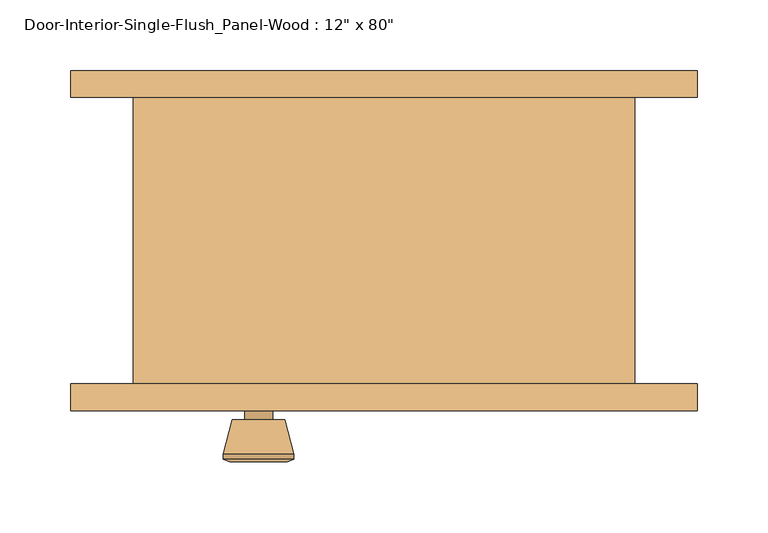
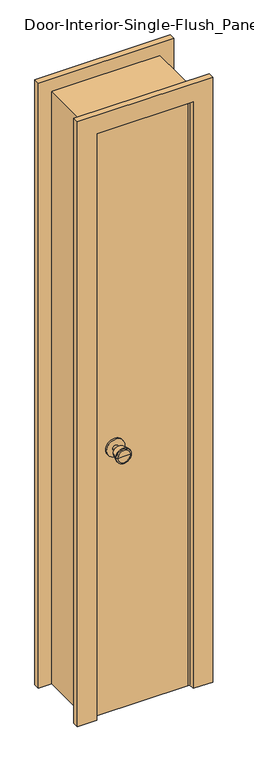
"""IFC4 building model written with IfcOpenShell, lengths in millimetres: door geometry."""

from ifc_helpers import new_model, si_unit, point, frame, frame_2d, origin, origin_with_axes, place, context, project, spatial, polyline, circle_curve, trimmed, segment, composite_curve, outline, extrude, faceted_brep, source, transform, mapped, element, save
from ifc_brep_helpers import plane_surface, cylinder_surface, revolved_surface, advanced_brep


def door_21b72c96(model_context):
    return source(origin(), model_context, "Body", "SolidModel", [
        advanced_brep(
        [(-88.9, -57.5, 914.4), (-98.9, -57.5, 914.4), (-78.9, -57.5, 914.4), (-68.4241324, -8.5, 914.4), (-109.3758676, -8.5, 914.4), (-88.9, -8.5, 914.4), (-63.9, -10.3278681, 914.4), (-113.9, -10.3278681, 914.4), (-63.9, -13.7915463, 914.4), (-113.9, -13.7915463, 914.4), (-70.263764, -38.5, 914.4), (-107.536236, -38.5, 914.4), (-78.9, -38.5, 914.4), (-98.9, -38.5, 914.4)],
        [
            (0, 1),
            (1, 2, circle_curve(frame((-88.9, -57.5, 914.4), z_axis=(0.0, -1.0, 0.0), x_axis=(-1.0, 0.0, 0.0)), 10.0)),
            (2, 0),
            (2, 1, circle_curve(frame((-88.9, -57.5, 914.4), z_axis=(0.0, -1.0, 0.0), x_axis=(-1.0, 0.0, 0.0)), 10.0)),
            (3, 4, circle_curve(frame((-88.9, -8.5, 914.4), z_axis=(0.0, 1.0, 0.0), x_axis=(-1.0, 0.0, 0.0)), 20.4758676)),
            (4, 5),
            (5, 3),
            (4, 3, circle_curve(frame((-88.9, -8.5, 914.4), z_axis=(0.0, 1.0, 0.0), x_axis=(-1.0, 0.0, 0.0)), 20.4758676)),
            (6, 7, circle_curve(frame((-88.9, -10.3278681, 914.4), z_axis=(0.0, 1.0, 0.0), x_axis=(-1.0, 0.0, 0.0)), 25.0)),
            (7, 4),
            (3, 6),
            (7, 6, circle_curve(frame((-88.9, -10.3278681, 914.4), z_axis=(0.0, 1.0, 0.0), x_axis=(-1.0, 0.0, 0.0)), 25.0)),
            (8, 9, circle_curve(frame((-88.9, -13.7915463, 914.4), z_axis=(0.0, 1.0, 0.0), x_axis=(-1.0, 0.0, 0.0)), 25.0)),
            (9, 7),
            (6, 8),
            (9, 8, circle_curve(frame((-88.9, -13.7915463, 914.4), z_axis=(0.0, 1.0, 0.0), x_axis=(-1.0, 0.0, 0.0)), 25.0)),
            (10, 11, circle_curve(frame((-88.9, -38.5, 914.4), z_axis=(0.0, 1.0, 0.0), x_axis=(-1.0, 0.0, 0.0)), 18.636236)),
            (11, 9),
            (8, 10),
            (11, 10, circle_curve(frame((-88.9, -38.5, 914.4), z_axis=(0.0, 1.0, 0.0), x_axis=(-1.0, 0.0, 0.0)), 18.636236)),
            (12, 13, circle_curve(frame((-88.9, -38.5, 914.4), z_axis=(0.0, 1.0, 0.0), x_axis=(-1.0, 0.0, 0.0)), 10.0)),
            (13, 11),
            (10, 12),
            (13, 12, circle_curve(frame((-88.9, -38.5, 914.4), z_axis=(0.0, 1.0, 0.0), x_axis=(-1.0, 0.0, 0.0)), 10.0)),
            (1, 13),
            (12, 2),
        ],
        [
            plane_surface(frame((-88.9, -57.5, 914.4), z_axis=(0.0, -1.0, 0.0), x_axis=(-1.0, 0.0, 0.0))),
            plane_surface(frame((-88.9, -8.5, 914.4), z_axis=(0.0, 1.0, 0.0), x_axis=(-1.0, 0.0, 0.0))),
            revolved_surface(polyline([(-109.3758676, -8.5, 914.4), (-113.9, -10.3278681, 914.4)]), (-88.9, -57.5, 914.4), (0.0, -1.0, 0.0)),
            cylinder_surface(frame((-88.9, -57.5, 914.4), z_axis=(0.0, -1.0, 0.0), x_axis=(-1.0, 0.0, 0.0)), 25.0),
            revolved_surface(polyline([(-113.9, -13.7915463, 914.4), (-107.536236, -38.5, 914.4)]), (-88.9, -57.5, 914.4), (0.0, -1.0, 0.0)),
            plane_surface(frame((-88.9, -38.5, 914.4), z_axis=(0.0, -1.0, 0.0), x_axis=(-1.0, 0.0, 0.0))),
            cylinder_surface(frame((-88.9, -57.5, 914.4), z_axis=(0.0, -1.0, 0.0), x_axis=(-1.0, 0.0, 0.0)), 10.0),
        ],
        [
            (0, [[1, 2, 3]]),
            (0, [[-3, 4, -1]]),
            (1, [[5, 6, 7]]),
            (1, [[8, -7, -6]]),
            (2, [[9, 10, -5, 11]]),
            (2, [[12, -11, -8, -10]]),
            (3, [[13, 14, -9, 15]]),
            (3, [[16, -15, -12, -14]]),
            (4, [[17, 18, -13, 19]]),
            (4, [[20, -19, -16, -18]]),
            (5, [[21, 22, -17, 23]]),
            (5, [[24, -23, -20, -22]]),
            (6, [[-2, 25, -21, 26]]),
            (6, [[-4, -26, -24, -25]]),
        ],
    ),
        extrude(outline(composite_curve([segment(trimmed(circle_curve(frame_2d((914.4, -88.9)), 30.0), [point((914.4, -118.9))], [point((914.4, -58.9))], False, "CARTESIAN"), True, "CONTINUOUS"), segment(trimmed(circle_curve(frame_2d((914.4, -88.9)), 30.0), [point((914.4, -58.9))], [point((914.4, -118.9))], False, "CARTESIAN"), True, "CONTINUOUS")], self_intersect=False)), frame((0.0, -63.5, 0.0), z_axis=(0.0, 1.0, 0.0), x_axis=(0.0, 0.0, 1.0)), (0.0, 0.0, 1.0), 6.0),
        advanced_brep(
        [(-88.9, -104.425, 914.4), (-78.9, -104.425, 914.4), (-98.9, -104.425, 914.4), (-68.4241324, -153.425, 914.4), (-88.9, -153.425, 914.4), (-109.3758676, -153.425, 914.4), (-63.9, -151.5971319, 914.4), (-113.9, -151.5971319, 914.4), (-63.9, -148.1334537, 914.4), (-113.9, -148.1334537, 914.4), (-70.263764, -123.425, 914.4), (-107.536236, -123.425, 914.4), (-78.9, -123.425, 914.4), (-98.9, -123.425, 914.4)],
        [
            (0, 1),
            (1, 2, circle_curve(frame((-88.9, -104.425, 914.4), z_axis=(0.0, 1.0, 0.0), x_axis=(-1.0, 0.0, 0.0)), 10.0)),
            (2, 0),
            (2, 1, circle_curve(frame((-88.9, -104.425, 914.4), z_axis=(0.0, 1.0, 0.0), x_axis=(-1.0, 0.0, 0.0)), 10.0)),
            (3, 4),
            (4, 5),
            (5, 3, circle_curve(frame((-88.9, -153.425, 914.4), z_axis=(0.0, -1.0, 0.0), x_axis=(-1.0, 0.0, 0.0)), 20.4758676)),
            (3, 5, circle_curve(frame((-88.9, -153.425, 914.4), z_axis=(0.0, -1.0, 0.0), x_axis=(-1.0, 0.0, 0.0)), 20.4758676)),
            (6, 3),
            (5, 7),
            (7, 6, circle_curve(frame((-88.9, -151.5971319, 914.4), z_axis=(0.0, -1.0, 0.0), x_axis=(-1.0, 0.0, 0.0)), 25.0)),
            (6, 7, circle_curve(frame((-88.9, -151.5971319, 914.4), z_axis=(0.0, -1.0, 0.0), x_axis=(-1.0, 0.0, 0.0)), 25.0)),
            (8, 6),
            (7, 9),
            (9, 8, circle_curve(frame((-88.9, -148.1334537, 914.4), z_axis=(0.0, -1.0, 0.0), x_axis=(-1.0, 0.0, 0.0)), 25.0)),
            (8, 9, circle_curve(frame((-88.9, -148.1334537, 914.4), z_axis=(0.0, -1.0, 0.0), x_axis=(-1.0, 0.0, 0.0)), 25.0)),
            (10, 8),
            (9, 11),
            (11, 10, circle_curve(frame((-88.9, -123.425, 914.4), z_axis=(0.0, -1.0, 0.0), x_axis=(-1.0, 0.0, 0.0)), 18.636236)),
            (10, 11, circle_curve(frame((-88.9, -123.425, 914.4), z_axis=(0.0, -1.0, 0.0), x_axis=(-1.0, 0.0, 0.0)), 18.636236)),
            (12, 10),
            (11, 13),
            (13, 12, circle_curve(frame((-88.9, -123.425, 914.4), z_axis=(0.0, -1.0, 0.0), x_axis=(-1.0, 0.0, 0.0)), 10.0)),
            (12, 13, circle_curve(frame((-88.9, -123.425, 914.4), z_axis=(0.0, -1.0, 0.0), x_axis=(-1.0, 0.0, 0.0)), 10.0)),
            (1, 12),
            (13, 2),
        ],
        [
            plane_surface(frame((-88.9, -104.425, 914.4), z_axis=(0.0, 1.0, 0.0), x_axis=(-1.0, 0.0, 0.0))),
            plane_surface(frame((-88.9, -153.425, 914.4), z_axis=(0.0, -1.0, 0.0), x_axis=(-1.0, 0.0, 0.0))),
            revolved_surface(polyline([(-109.3758676, -153.425, 914.4), (-113.9, -151.5971319, 914.4)]), (-88.9, -104.425, 914.4), (0.0, 1.0, 0.0)),
            cylinder_surface(frame((-88.9, -104.425, 914.4), z_axis=(0.0, 1.0, 0.0), x_axis=(-1.0, 0.0, 0.0)), 25.0),
            revolved_surface(polyline([(-113.9, -148.1334537, 914.4), (-107.536236, -123.425, 914.4)]), (-88.9, -104.425, 914.4), (0.0, 1.0, 0.0)),
            plane_surface(frame((-88.9, -123.425, 914.4), z_axis=(0.0, 1.0, 0.0), x_axis=(-1.0, 0.0, 0.0))),
            cylinder_surface(frame((-88.9, -104.425, 914.4), z_axis=(0.0, 1.0, 0.0), x_axis=(-1.0, 0.0, 0.0)), 10.0),
        ],
        [
            (0, [[1, 2, 3]]),
            (0, [[-3, 4, -1]]),
            (1, [[5, 6, 7]]),
            (1, [[-6, -5, 8]]),
            (2, [[9, -7, 10, 11]]),
            (2, [[-10, -8, -9, 12]]),
            (3, [[13, -11, 14, 15]]),
            (3, [[-14, -12, -13, 16]]),
            (4, [[17, -15, 18, 19]]),
            (4, [[-18, -16, -17, 20]]),
            (5, [[21, -19, 22, 23]]),
            (5, [[-22, -20, -21, 24]]),
            (6, [[25, -23, 26, -2]]),
            (6, [[-26, -24, -25, -4]]),
        ],
    ),
        extrude(outline(composite_curve([segment(trimmed(circle_curve(frame_2d((914.4, -88.9)), 30.0), [point((914.4, -118.9))], [point((914.4, -58.9))], False, "CARTESIAN"), True, "CONTINUOUS"), segment(trimmed(circle_curve(frame_2d((914.4, -88.9)), 30.0), [point((914.4, -58.9))], [point((914.4, -118.9))], False, "CARTESIAN"), True, "CONTINUOUS")], self_intersect=False)), frame((0.0, -104.425, 0.0), z_axis=(0.0, 1.0, 0.0), x_axis=(0.0, 0.0, 1.0)), (0.0, 0.0, 1.0), 6.0),
        extrude(outline(polyline([(152.4, -63.5), (152.4, -98.425), (-152.4, -98.425), (-152.4, -63.5), (152.4, -63.5)])), origin_with_axes(), (0.0, 0.0, 1.0), 2032.0),
        faceted_brep([(177.8, -98.425, 0.0), (152.4, -98.425, 0.0), (152.4, -63.5, 0.0), (139.7, -63.5, 0.0), (139.7, -28.575, 0.0), (152.4, -28.575, 0.0), (152.4, 104.775, 0.0), (177.8, 104.775, 0.0), (177.8, 104.775, 2057.4), (177.8, -98.425, 2057.4), (152.4, 104.775, 2032.0), (-152.4, 104.775, 2032.0), (-152.4, 104.775, 0.0), (-177.8, 104.775, 0.0), (-177.8, 104.775, 2057.4), (152.4, -28.575, 2032.0), (139.7, -28.575, 2019.3), (-139.7, -28.575, 2019.3), (-139.7, -28.575, 0.0), (-152.4, -28.575, 0.0), (-152.4, -28.575, 2032.0), (139.7, -63.5, 2019.3), (152.4, -63.5, 2032.0), (-152.4, -63.5, 2032.0), (-152.4, -63.5, 0.0), (-139.7, -63.5, 0.0), (-139.7, -63.5, 2019.3), (152.4, -98.425, 2032.0), (-177.8, -98.425, 2057.4), (-177.8, -98.425, 0.0), (-152.4, -98.425, 0.0), (-152.4, -98.425, 2032.0)], [[[0, 1, 2, 3, 4, 5, 6, 7]], [[7, 8, 9, 0]], [[6, 10, 11, 12, 13, 14, 8, 7]], [[5, 15, 10, 6]], [[4, 16, 17, 18, 19, 20, 15, 5]], [[3, 21, 16, 4]], [[2, 22, 23, 24, 25, 26, 21, 3]], [[1, 27, 22, 2]], [[0, 9, 28, 29, 30, 31, 27, 1]], [[8, 14, 28, 9]], [[15, 20, 11, 10]], [[21, 26, 17, 16]], [[27, 31, 23, 22]], [[29, 13, 12, 19, 18, 25, 24, 30]], [[14, 13, 29, 28]], [[20, 19, 12, 11]], [[26, 25, 18, 17]], [[31, 30, 24, 23]]]),
        extrude(outline(polyline([(0.0, 222.25), (2101.85, 222.25), (2101.85, -222.25), (0.0, -222.25), (0.0, -158.75), (2038.35, -158.75), (2038.35, 158.75), (0.0, 158.75), (0.0, 222.25)])), frame((0.0, 104.775, 0.0), z_axis=(0.0, 1.0, 0.0), x_axis=(0.0, 0.0, 1.0)), (0.0, 0.0, 1.0), 19.05),
        extrude(outline(polyline([(0.0, 222.25), (2101.85, 222.25), (2101.85, -222.25), (0.0, -222.25), (0.0, -158.75), (2038.35, -158.75), (2038.35, 158.75), (0.0, 158.75), (0.0, 222.25)])), frame((0.0, -117.475, 0.0), z_axis=(0.0, 1.0, 0.0), x_axis=(0.0, 0.0, 1.0)), (0.0, 0.0, 1.0), 19.05),
    ])


if __name__ == "__main__":
    model = new_model("IFC4")
    model_context = context("Model", 3, world=origin())
    ifc_project = project(units=[si_unit("LENGTHUNIT", "METRE", prefix="MILLI")], contexts=[model_context])
    site = spatial("IfcSite", under=ifc_project)
    building = spatial("IfcBuilding", under=site)
    placement = place(None, origin())
    door_shape = door_21b72c96(model_context)
    element("IfcDoor", 1, ObjectType="Door-Interior-Single-Flush_Panel-Wood : 12\" x 80\"", at=placement, inside=building, context=model_context, shape_type="MappedRepresentation", body=[
        mapped(door_shape, transform((0.0, 0.0, 0.0), x_axis=(1.0, 0.0, 0.0), y_axis=(0.0, 1.0, 0.0), z_axis=(0.0, 0.0, 1.0))),
    ])
    save(model, "model.ifc")

# Revit data of these elements
# Type "Door-Interior-Single-Flush_Panel-Wood : 12\" x 80\""
#   Type Mark = "10"
#   Assembly Code = "C1020300"
#   Analytic Construction = "Wooden"
#   Thickness = 0' - 1 3/8"
#   Thermal Resistance (R) = 2.5876 (h·ft²·°F)/BTU
#   Swing Angle [instance default] = 90.00°
#   Rough Width = 1' - 2"
#   Rough Height = 6' - 9"
#   Height = 6' - 8"
#   Width = 1' - 0"
#   Heat Transfer Coefficient (U) = 0.3865 BTU/(h·ft²·°F)
#   Trim Material = Cherry
#   Panel Material = Cherry
#   Frame Material = Cherry
#   Door Handle Material = Aluminum
#   Visual Light Transmittance = 0
#   Solar Heat Gain Coefficient = 0
#   Wall Closure = (empty or 0)
#   Function = (empty or 0)
# Element 1 (IfcDoor, "Door-Interior-Single-Flush_Panel-Wood : 12\" x 80\"")
#   Materials on its faces: "Cherry", "Aluminum"
# Materials
#   "Cherry": class "Wood", colour RGB 226 177 128, transparency 0, Description = "Prunus Serotina", Cost = 0
#   "Aluminum": class "Metal", colour RGB 247 247 247, transparency 0, Description = "Aluminum 6061", Cost = 0
